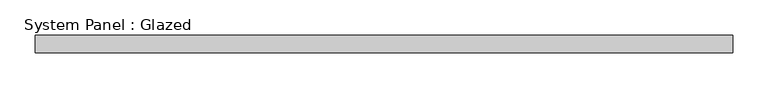
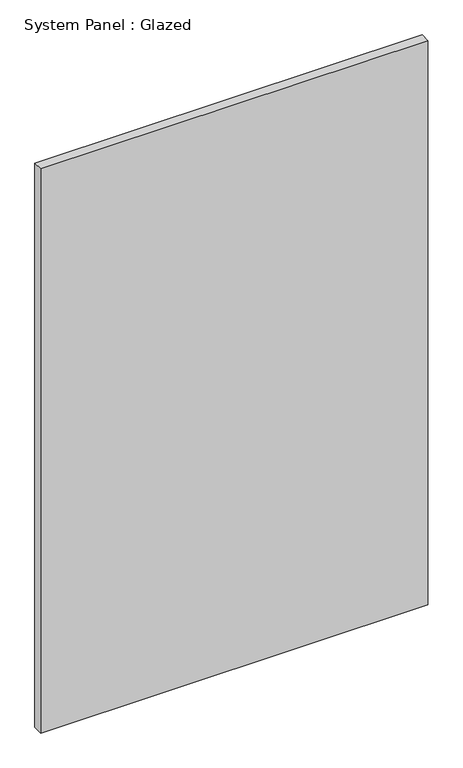
"""IFC4 building model written with IfcOpenShell, lengths in millimetres: plate geometry, System Panel : Glazed."""

from ifc_helpers import new_model, si_unit, origin, origin_with_axes, place, context, project, spatial, polyline, outline, extrude, source, transform, mapped, element, save


def system_panel_glazed_fc0c7c09(model_context):
    return source(origin(), model_context, "Body", "SweptSolid", [
        extrude(outline(polyline([(498.475, 19.05), (-498.475, 19.05), (-498.475, 44.45), (498.475, 44.45), (498.475, 19.05)])), origin_with_axes(), (0.0, 0.0, 1.0), 1535.7829369),
    ])


if __name__ == "__main__":
    model = new_model("IFC4")
    model_context = context("Model", 3, world=origin())
    ifc_project = project(units=[si_unit("LENGTHUNIT", "METRE", prefix="MILLI")], contexts=[model_context])
    site = spatial("IfcSite", under=ifc_project)
    building = spatial("IfcBuilding", under=site)
    placement = place(None, origin())
    system_panel_glazed_shape = system_panel_glazed_fc0c7c09(model_context)
    element("IfcPlate", 1, ObjectType="System Panel : Glazed", at=placement, inside=building, context=model_context, shape_type="MappedRepresentation", body=[
        mapped(system_panel_glazed_shape, transform((0.0, 0.0, 0.0), x_axis=(1.0, 0.0, 0.0), y_axis=(0.0, 1.0, 0.0), z_axis=(0.0, 0.0, 1.0))),
    ])
    save(model, "model.ifc")

# Revit data of these elements
# Type "System Panel : Glazed"
#   Construction Type Id = "GSP4R"
#   Analytic Construction = "1/8 in Pilkington single glazing"
#   Visual Light Transmittance = 0.9
#   Solar Heat Gain Coefficient = 0.86
#   Heat Transfer Coefficient (U) = 1.18115 BTU/(h·ft²·°F)
#   Define Thermal Properties by = 1
# Element 1 (IfcPlate, "System Panel : Glazed")
#   Materials on its faces: "Glass"
# Materials
#   "Glass": class "Glass", colour RGB 0 128 192, transparency 0.75, Description = "Soda Lime Glass", Cost = 0
